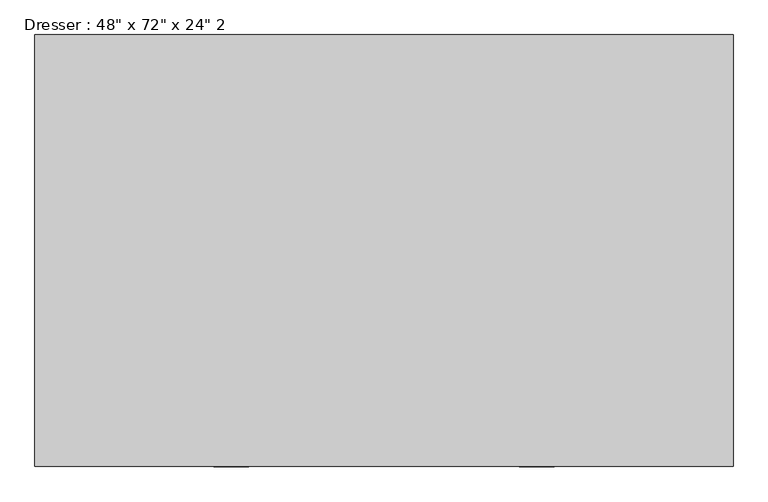
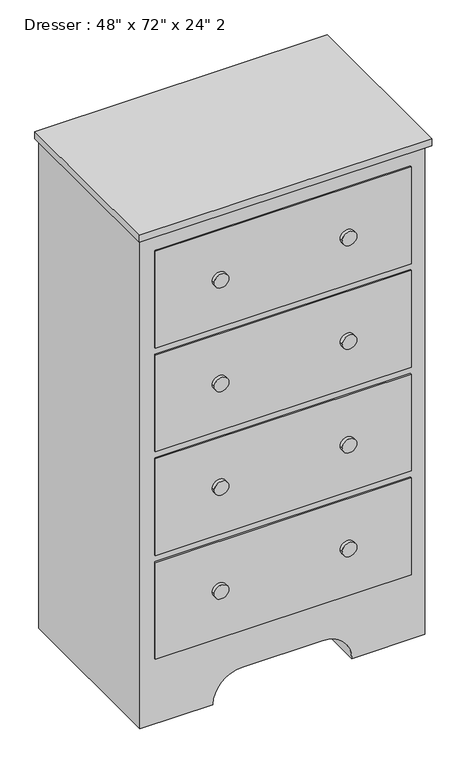
"""IFC4 building model written with IfcOpenShell, lengths in millimetres: furniture geometry."""

from ifc_helpers import new_model, si_unit, point, frame, frame_2d, origin, place, context, project, spatial, polyline, circle_curve, trimmed, segment, composite_curve, outline, extrude, source, transform, mapped, element, save


def furniture_f13f95b7(model_context):
    return source(origin(), model_context, "Body", "SweptSolid", [
        extrude(outline(polyline([(238.8067402, -58.3629541), (238.8067402, -687.0129541), (-777.1932598, -687.0129541), (-777.1932598, -58.3629541), (238.8067402, -58.3629541)])), frame((0.0, 0.0, 1803.4), z_axis=(0.0, 0.0, 1.0), x_axis=(1.0, 0.0, 0.0)), (0.0, 0.0, 1.0), 25.4),
        extrude(outline(composite_curve([segment(polyline([(0.0, 226.1067402), (1803.4, 226.1067402), (1803.4, -764.4932598), (0.0, -764.4932598), (0.0, -510.4932598)]), True, "CONTINUOUS"), segment(trimmed(circle_curve(frame_2d((0.0, -408.8932598)), 101.6), [point((0.0, -510.4932598))], [point((101.6, -408.8932598))], True, "CARTESIAN"), True, "CONTINUOUS"), segment(polyline([(101.6, -408.8932598), (101.6, -129.4932598)]), True, "CONTINUOUS"), segment(trimmed(circle_curve(frame_2d((0.0, -129.4932598)), 101.6), [point((101.6, -129.4932598))], [point((0.0, -27.8932598))], True, "CARTESIAN"), True, "CONTINUOUS"), segment(polyline([(0.0, -27.8932598), (0.0, 226.1067402)]), True, "CONTINUOUS")], self_intersect=False)), frame((0.0, -667.9629541, 0.0), z_axis=(0.0, 1.0, 0.0), x_axis=(0.0, 0.0, 1.0)), (0.0, 0.0, 1.0), 609.6),
        extrude(outline(composite_curve([segment(trimmed(circle_curve(frame_2d((1562.1, -46.9432598)), 25.4), [point((1562.1, -72.3432598))], [point((1562.1, -21.5432598))], False, "CARTESIAN"), True, "CONTINUOUS"), segment(trimmed(circle_curve(frame_2d((1562.1, -46.9432598)), 25.4), [point((1562.1, -21.5432598))], [point((1562.1, -72.3432598))], False, "CARTESIAN"), True, "CONTINUOUS")], self_intersect=False)), frame((0.0, -687.0129541, 0.0), z_axis=(0.0, 1.0, 0.0), x_axis=(0.0, 0.0, 1.0)), (0.0, 0.0, 1.0), 12.7),
        extrude(outline(composite_curve([segment(trimmed(circle_curve(frame_2d((1181.1, -46.9432598)), 25.4), [point((1181.1, -72.3432598))], [point((1181.1, -21.5432598))], False, "CARTESIAN"), True, "CONTINUOUS"), segment(trimmed(circle_curve(frame_2d((1181.1, -46.9432598)), 25.4), [point((1181.1, -21.5432598))], [point((1181.1, -72.3432598))], False, "CARTESIAN"), True, "CONTINUOUS")], self_intersect=False)), frame((0.0, -687.0129541, 0.0), z_axis=(0.0, 1.0, 0.0), x_axis=(0.0, 0.0, 1.0)), (0.0, 0.0, 1.0), 12.7),
        extrude(outline(composite_curve([segment(trimmed(circle_curve(frame_2d((800.1, -46.9432598)), 25.4), [point((800.1, -72.3432598))], [point((800.1, -21.5432598))], False, "CARTESIAN"), True, "CONTINUOUS"), segment(trimmed(circle_curve(frame_2d((800.1, -46.9432598)), 25.4), [point((800.1, -21.5432598))], [point((800.1, -72.3432598))], False, "CARTESIAN"), True, "CONTINUOUS")], self_intersect=False)), frame((0.0, -687.0129541, 0.0), z_axis=(0.0, 1.0, 0.0), x_axis=(0.0, 0.0, 1.0)), (0.0, 0.0, 1.0), 12.7),
        extrude(outline(composite_curve([segment(trimmed(circle_curve(frame_2d((419.1, -46.9432598)), 25.4), [point((419.1, -72.3432598))], [point((419.1, -21.5432598))], False, "CARTESIAN"), True, "CONTINUOUS"), segment(trimmed(circle_curve(frame_2d((419.1, -46.9432598)), 25.4), [point((419.1, -21.5432598))], [point((419.1, -72.3432598))], False, "CARTESIAN"), True, "CONTINUOUS")], self_intersect=False)), frame((0.0, -687.0129541, 0.0), z_axis=(0.0, 1.0, 0.0), x_axis=(0.0, 0.0, 1.0)), (0.0, 0.0, 1.0), 12.7),
        extrude(outline(composite_curve([segment(trimmed(circle_curve(frame_2d((419.1, -491.4432598)), 25.4), [point((419.1, -516.8432598))], [point((419.1, -466.0432598))], False, "CARTESIAN"), True, "CONTINUOUS"), segment(trimmed(circle_curve(frame_2d((419.1, -491.4432598)), 25.4), [point((419.1, -466.0432598))], [point((419.1, -516.8432598))], False, "CARTESIAN"), True, "CONTINUOUS")], self_intersect=False)), frame((0.0, -687.0129541, 0.0), z_axis=(0.0, 1.0, 0.0), x_axis=(0.0, 0.0, 1.0)), (0.0, 0.0, 1.0), 12.7),
        extrude(outline(composite_curve([segment(trimmed(circle_curve(frame_2d((800.1, -491.4432598)), 25.4), [point((800.1, -516.8432598))], [point((800.1, -466.0432598))], False, "CARTESIAN"), True, "CONTINUOUS"), segment(trimmed(circle_curve(frame_2d((800.1, -491.4432598)), 25.4), [point((800.1, -466.0432598))], [point((800.1, -516.8432598))], False, "CARTESIAN"), True, "CONTINUOUS")], self_intersect=False)), frame((0.0, -687.0129541, 0.0), z_axis=(0.0, 1.0, 0.0), x_axis=(0.0, 0.0, 1.0)), (0.0, 0.0, 1.0), 12.7),
        extrude(outline(composite_curve([segment(trimmed(circle_curve(frame_2d((1181.1, -491.4432598)), 25.4), [point((1181.1, -516.8432598))], [point((1181.1, -466.0432598))], False, "CARTESIAN"), True, "CONTINUOUS"), segment(trimmed(circle_curve(frame_2d((1181.1, -491.4432598)), 25.4), [point((1181.1, -466.0432598))], [point((1181.1, -516.8432598))], False, "CARTESIAN"), True, "CONTINUOUS")], self_intersect=False)), frame((0.0, -687.0129541, 0.0), z_axis=(0.0, 1.0, 0.0), x_axis=(0.0, 0.0, 1.0)), (0.0, 0.0, 1.0), 12.7),
        extrude(outline(composite_curve([segment(trimmed(circle_curve(frame_2d((1562.1, -491.4432598)), 25.4), [point((1562.1, -516.8432598))], [point((1562.1, -466.0432598))], False, "CARTESIAN"), True, "CONTINUOUS"), segment(trimmed(circle_curve(frame_2d((1562.1, -491.4432598)), 25.4), [point((1562.1, -466.0432598))], [point((1562.1, -516.8432598))], False, "CARTESIAN"), True, "CONTINUOUS")], self_intersect=False)), frame((0.0, -687.0129541, 0.0), z_axis=(0.0, 1.0, 0.0), x_axis=(0.0, 0.0, 1.0)), (0.0, 0.0, 1.0), 12.7),
        extrude(outline(polyline([(175.3067402, -674.3129541), (-713.6932598, -674.3129541), (-713.6932598, -667.9629541), (175.3067402, -667.9629541), (175.3067402, -674.3129541)])), frame((0.0, 0.0, 1384.3), z_axis=(0.0, 0.0, 1.0), x_axis=(1.0, 0.0, 0.0)), (0.0, 0.0, 1.0), 355.6),
        extrude(outline(polyline([(175.3067402, -674.3129541), (-713.6932598, -674.3129541), (-713.6932598, -667.9629541), (175.3067402, -667.9629541), (175.3067402, -674.3129541)])), frame((0.0, 0.0, 1003.3), z_axis=(0.0, 0.0, 1.0), x_axis=(1.0, 0.0, 0.0)), (0.0, 0.0, 1.0), 355.6),
        extrude(outline(polyline([(175.3067402, -674.3129541), (-713.6932598, -674.3129541), (-713.6932598, -667.9629541), (175.3067402, -667.9629541), (175.3067402, -674.3129541)])), frame((0.0, 0.0, 622.3), z_axis=(0.0, 0.0, 1.0), x_axis=(1.0, 0.0, 0.0)), (0.0, 0.0, 1.0), 355.6),
        extrude(outline(polyline([(175.3067402, -674.3129541), (-713.6932598, -674.3129541), (-713.6932598, -667.9629541), (175.3067402, -667.9629541), (175.3067402, -674.3129541)])), frame((0.0, 0.0, 241.3), z_axis=(0.0, 0.0, 1.0), x_axis=(1.0, 0.0, 0.0)), (0.0, 0.0, 1.0), 355.6),
    ])


if __name__ == "__main__":
    model = new_model("IFC4")
    model_context = context("Model", 3, world=origin())
    ifc_project = project(units=[si_unit("LENGTHUNIT", "METRE", prefix="MILLI")], contexts=[model_context])
    site = spatial("IfcSite", under=ifc_project)
    building = spatial("IfcBuilding", under=site)
    placement = place(None, origin())
    furniture_shape = furniture_f13f95b7(model_context)
    element("IfcFurniture", 1, ObjectType="Dresser : 48\" x 72\" x 24\" 2", at=placement, inside=building, context=model_context, shape_type="MappedRepresentation", body=[
        mapped(furniture_shape, transform((0.0, 0.0, 0.0), x_axis=(1.0, 0.0, 0.0), y_axis=(0.0, 1.0, 0.0), z_axis=(0.0, 0.0, 1.0))),
    ])
    save(model, "model.ifc")

# Revit data of these elements
# Type "Dresser : 48\" x 72\" x 24\" 2"
#   Assembly Code = "E2020200"
#   Depth = 2' - 0"
#   Height = 6' - 0"
#   Width = 3' - 3"
#   Dresser Material = Wood Door Panel - Birch
#   Drawer Material = Wood Door Panel - Birch
#   Knob Material = Cherry
#   Default Elevation = 0
# Element 1 (IfcFurniture, "Dresser : 48\" x 72\" x 24\" 2")
#   Materials on its faces: "Laminate, Ivory, Matte", "Cherry", "Wood Door Panel - Birch"
# Materials
#   "Wood Door Panel - Birch": class "Wood", colour RGB 166 116 52, transparency 0
#   "Cherry": class "Wood", colour RGB 226 177 128, transparency 0, Description = "Prunus Serotina", Cost = 0
#   "Laminate, Ivory, Matte": class "Plastic", colour RGB 247 247 239, transparency 0, Description = "Plastic Laminate - Ivory, Matte", Cost = 0
